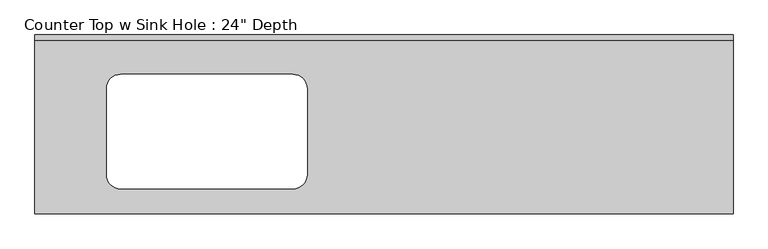
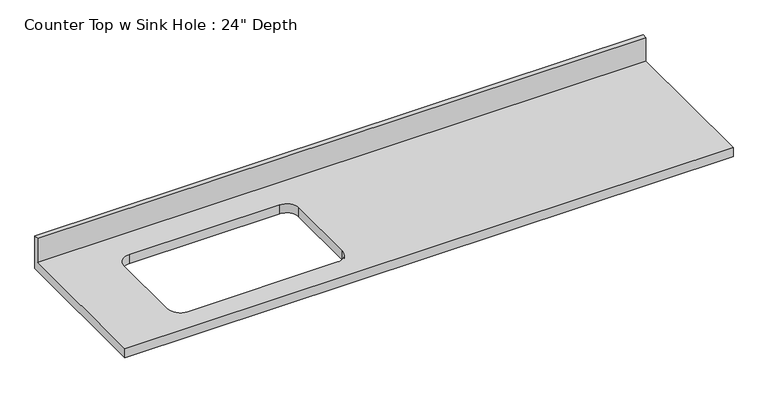
"""IFC4 building model written with IfcOpenShell, lengths in millimetres: furniture geometry."""

from ifc_helpers import new_model, si_unit, frame, origin, place, context, project, spatial, polyline, circle_curve, source, transform, mapped, element, save
from ifc_brep_helpers import plane_surface, revolved_surface, advanced_brep


def furniture_d3a4b1a9(model_context):
    return source(origin(), model_context, "Body", "AdvancedBrep", [
        advanced_brep(
        [(-1200.4622951, -635.0, 914.4), (1276.0377049, -635.0, 914.4), (1276.0377049, -19.05, 914.4), (-1200.4622951, -19.05, 914.4), (-895.6622951, -139.7, 914.4), (-286.0622951, -139.7, 914.4), (-235.2622951, -190.5, 914.4), (-235.2622951, -495.3, 914.4), (-286.0622951, -546.1, 914.4), (-895.6622951, -546.1, 914.4), (-946.4622951, -495.3, 914.4), (-946.4622951, -190.5, 914.4), (1276.0377049, 0.0, 876.3), (1276.0377049, -635.0, 876.3), (-1200.4622951, -635.0, 876.3), (-1200.4622951, 0.0, 876.3), (-286.0622951, -139.7, 876.3), (-895.6622951, -139.7, 876.3), (-946.4622951, -190.5, 876.3), (-946.4622951, -495.3, 876.3), (-895.6622951, -546.1, 876.3), (-286.0622951, -546.1, 876.3), (-235.2622951, -495.3, 876.3), (-235.2622951, -190.5, 876.3), (-1200.4622951, 0.0, 1016.0), (1276.0377049, 0.0, 1016.0), (-1200.4622951, -19.05, 1016.0), (1276.0377049, -19.05, 1016.0)],
        [
            (0, 1),
            (1, 2),
            (2, 3),
            (3, 0),
            (4, 5),
            (5, 6, circle_curve(frame((-286.0622951, -190.5, 914.4), z_axis=(0.0, 0.0, -1.0), x_axis=(1.0, 0.0, 0.0)), 50.8)),
            (6, 7),
            (7, 8, circle_curve(frame((-286.0622951, -495.3, 914.4), z_axis=(0.0, 0.0, -1.0), x_axis=(1.0, 0.0, 0.0)), 50.8)),
            (8, 9),
            (9, 10, circle_curve(frame((-895.6622951, -495.3, 914.4), z_axis=(0.0, 0.0, -1.0), x_axis=(1.0, 0.0, 0.0)), 50.8)),
            (10, 11),
            (11, 4, circle_curve(frame((-895.6622951, -190.5, 914.4), z_axis=(0.0, 0.0, -1.0), x_axis=(1.0, 0.0, 0.0)), 50.8)),
            (12, 13),
            (13, 14),
            (14, 15),
            (15, 12),
            (16, 17),
            (17, 18, circle_curve(frame((-895.6622951, -190.5, 876.3), z_axis=(0.0, 0.0, 1.0), x_axis=(1.0, 0.0, 0.0)), 50.8)),
            (18, 19),
            (19, 20, circle_curve(frame((-895.6622951, -495.3, 876.3), z_axis=(0.0, 0.0, 1.0), x_axis=(1.0, 0.0, 0.0)), 50.8)),
            (20, 21),
            (21, 22, circle_curve(frame((-286.0622951, -495.3, 876.3), z_axis=(0.0, 0.0, 1.0), x_axis=(1.0, 0.0, 0.0)), 50.8)),
            (22, 23),
            (23, 16, circle_curve(frame((-286.0622951, -190.5, 876.3), z_axis=(0.0, 0.0, 1.0), x_axis=(1.0, 0.0, 0.0)), 50.8)),
            (15, 24),
            (24, 25),
            (25, 12),
            (14, 0),
            (3, 26),
            (26, 24),
            (13, 1),
            (25, 27),
            (27, 2),
            (26, 27),
            (4, 17),
            (16, 5),
            (11, 18),
            (10, 19),
            (9, 20),
            (8, 21),
            (7, 22),
            (6, 23),
        ],
        [
            plane_surface(frame((-1200.4622951, 0.0, 914.4), z_axis=(0.0, 0.0, 1.0), x_axis=(-1.0, 0.0, 0.0))),
            plane_surface(frame((-1200.4622951, 0.0, 876.3), z_axis=(0.0, 0.0, -1.0), x_axis=(1.0, 0.0, 0.0))),
            plane_surface(frame((1276.0377049, 0.0, 914.4), z_axis=(0.0, 1.0, 0.0), x_axis=(0.0, 0.0, -1.0))),
            plane_surface(frame((-1200.4622951, 0.0, 914.4), z_axis=(-1.0, 0.0, 0.0), x_axis=(0.0, 0.0, -1.0))),
            plane_surface(frame((-1200.4622951, -635.0, 914.4), z_axis=(0.0, -1.0, 0.0), x_axis=(0.0, 0.0, -1.0))),
            plane_surface(frame((1276.0377049, -635.0, 914.4), z_axis=(1.0, 0.0, 0.0), x_axis=(0.0, 0.0, -1.0))),
            plane_surface(frame((-1200.4622951, 0.0, 1016.0), z_axis=(0.0, 0.0, 1.0), x_axis=(0.0, -1.0, 0.0))),
            plane_surface(frame((-1200.4622951, -19.05, 1016.0), z_axis=(0.0, -1.0, 0.0), x_axis=(0.0, 0.0, -1.0))),
            plane_surface(frame((-286.0622951, -139.7, 914.4), z_axis=(0.0, -1.0, 0.0), x_axis=(0.0, 0.0, -1.0))),
            revolved_surface(polyline([(-844.8622951000001, -190.5, 914.4), (-844.8622951000001, -190.5, 876.3)]), (-895.6622951, -190.5, 876.3), (0.0, 0.0, 1.0)),
            plane_surface(frame((-946.4622951, -190.5, 914.4), z_axis=(1.0, 0.0, 0.0), x_axis=(0.0, 0.0, -1.0))),
            revolved_surface(polyline([(-844.8622951000001, -495.3, 914.4), (-844.8622951000001, -495.3, 876.3)]), (-895.6622951, -495.3, 876.3), (0.0, 0.0, 1.0)),
            plane_surface(frame((-895.6622951, -546.1, 914.4), z_axis=(0.0, 1.0, 0.0), x_axis=(0.0, 0.0, -1.0))),
            revolved_surface(polyline([(-235.26229509999996, -495.3, 914.4), (-235.26229509999996, -495.3, 876.3)]), (-286.0622951, -495.3, 876.3), (0.0, 0.0, 1.0)),
            plane_surface(frame((-235.2622951, -495.3, 914.4), z_axis=(-1.0, 0.0, 0.0), x_axis=(0.0, 0.0, -1.0))),
            revolved_surface(polyline([(-235.26229509999996, -190.5, 914.4), (-235.26229509999996, -190.5, 876.3)]), (-286.0622951, -190.5, 876.3), (0.0, 0.0, 1.0)),
        ],
        [
            (0, [[1, 2, 3, 4], [5, 6, 7, 8, 9, 10, 11, 12]]),
            (1, [[13, 14, 15, 16], [17, 18, 19, 20, 21, 22, 23, 24]]),
            (2, [[-16, 25, 26, 27]]),
            (3, [[-15, 28, -4, 29, 30, -25]]),
            (4, [[-1, -28, -14, 31]]),
            (5, [[-13, -27, 32, 33, -2, -31]]),
            (6, [[-30, 34, -32, -26]]),
            (7, [[-34, -29, -3, -33]]),
            (8, [[35, -17, 36, -5]]),
            (9, [[-35, -12, 37, -18]]),
            (10, [[-37, -11, 38, -19]]),
            (11, [[-38, -10, 39, -20]]),
            (12, [[-39, -9, 40, -21]]),
            (13, [[-40, -8, 41, -22]]),
            (14, [[-41, -7, 42, -23]]),
            (15, [[-36, -24, -42, -6]]),
        ],
    ),
    ])


if __name__ == "__main__":
    model = new_model("IFC4")
    model_context = context("Model", 3, world=origin())
    ifc_project = project(units=[si_unit("LENGTHUNIT", "METRE", prefix="MILLI")], contexts=[model_context])
    site = spatial("IfcSite", under=ifc_project)
    building = spatial("IfcBuilding", under=site)
    placement = place(None, origin())
    furniture_shape = furniture_d3a4b1a9(model_context)
    element("IfcFurniture", 1, ObjectType="Counter Top w Sink Hole : 24\" Depth", at=placement, inside=building, context=model_context, shape_type="MappedRepresentation", body=[
        mapped(furniture_shape, transform((0.0, 0.0, 0.0), x_axis=(1.0, 0.0, 0.0), y_axis=(0.0, 1.0, 0.0), z_axis=(0.0, 0.0, 1.0))),
    ])
    save(model, "model.ifc")

# Revit data of these elements
# Type "Counter Top w Sink Hole : 24\" Depth"
#   Assembly Code = "C1030400"
#   Counter Thickness = 0' - 1 1/2"
#   Depth = 2' - 1"
#   Height = 3' - 0"
#   Length [instance default] = 8' - 0"
#   Sink Location [instance default] = 2' - 0"
#   Sink Location To Wall [instance default] = 0' - 6"
#   Sink Opening Depth [instance default] = 1' - 3"
#   Sink Opening Width [instance default] = 2' - 3"
#   Counter Top Material = none
#   Default Elevation = 0
# Element 1 (IfcFurniture, "Counter Top w Sink Hole : 24\" Depth")
#   Length = 8' - 1 1/2"
#   Materials on its faces: "Counter Top"
# Materials
#   "Counter Top": class "Wood", colour RGB 226 177 128, transparency 0
